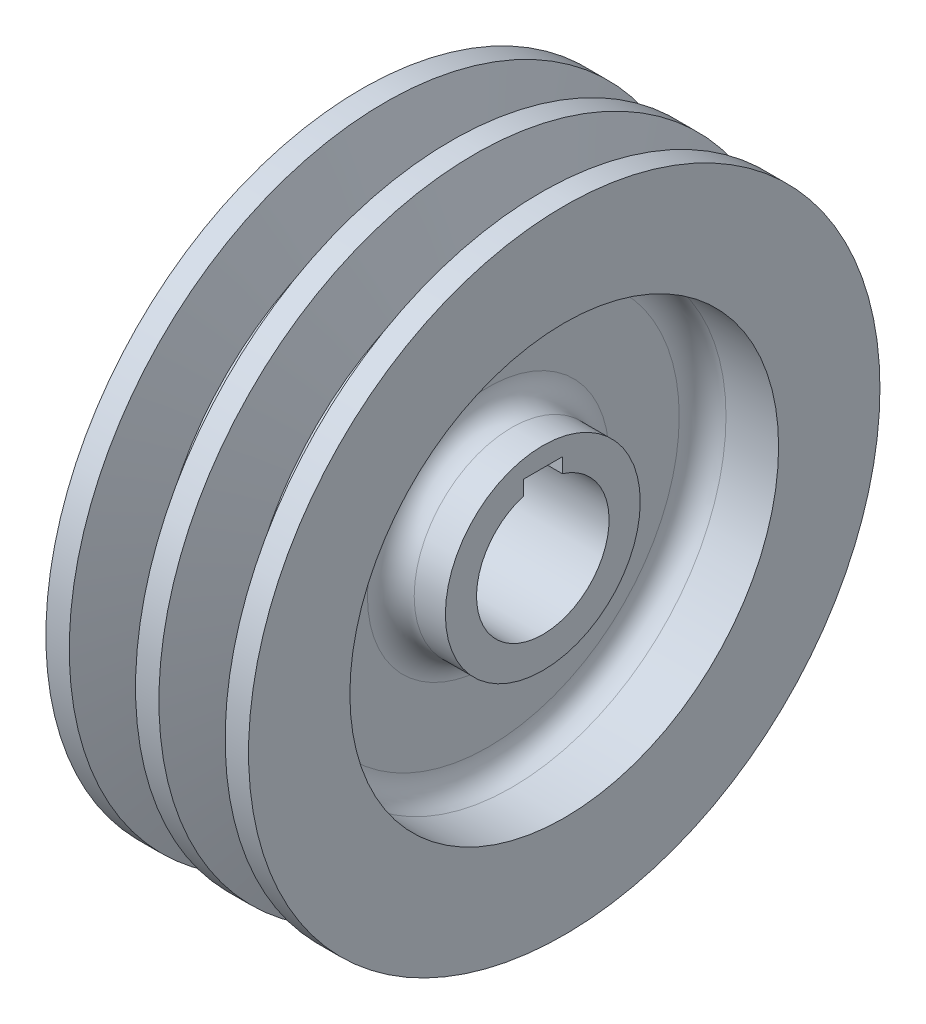
ISO-10303-21;
HEADER;
FILE_DESCRIPTION(('STEP AP214'),'2;1');
FILE_NAME('part.step','',(''),(''),'','','');
FILE_SCHEMA(('AUTOMOTIVE_DESIGN { 1 0 10303 214 1 1 1 1 }'));
ENDSEC;
DATA;
#1=APPLICATION_CONTEXT('core data for automotive mechanical design processes');
#2=APPLICATION_PROTOCOL_DEFINITION('international standard','automotive_design',2000,#1);
#3=PRODUCT_CONTEXT('',#1,'mechanical');
#4=PRODUCT('Part','Part','',(#3));
#5=PRODUCT_RELATED_PRODUCT_CATEGORY('part','',(#4));
#6=PRODUCT_DEFINITION_FORMATION('','',#4);
#7=PRODUCT_DEFINITION_CONTEXT('part definition',#1,'design');
#8=PRODUCT_DEFINITION('design','',#6,#7);
#9=PRODUCT_DEFINITION_SHAPE('','',#8);
#10=(LENGTH_UNIT() NAMED_UNIT(*) SI_UNIT(.MILLI.,.METRE.));
#11=(NAMED_UNIT(*) PLANE_ANGLE_UNIT() SI_UNIT($,.RADIAN.));
#12=(NAMED_UNIT(*) SI_UNIT($,.STERADIAN.) SOLID_ANGLE_UNIT());
#13=UNCERTAINTY_MEASURE_WITH_UNIT(LENGTH_MEASURE(1.E-05),#10,'distance_accuracy_value','');
#14=(GEOMETRIC_REPRESENTATION_CONTEXT(3) GLOBAL_UNCERTAINTY_ASSIGNED_CONTEXT((#13)) GLOBAL_UNIT_ASSIGNED_CONTEXT((#10,
#11,#12)) REPRESENTATION_CONTEXT('',''));
#15=CARTESIAN_POINT('',(0.,0.,0.));
#16=DIRECTION('',(0.,0.,1.));
#17=DIRECTION('',(1.,0.,0.));
#18=AXIS2_PLACEMENT_3D('',#15,#16,#17);
#19=CARTESIAN_POINT('',(52.,0.,0.));
#20=DIRECTION('',(-1.,0.,0.));
#21=DIRECTION('',(0.,0.,1.));
#22=AXIS2_PLACEMENT_3D('',#19,#20,#21);
#23=PLANE('',#22);
#24=CARTESIAN_POINT('',(52.,0.,0.));
#25=DIRECTION('',(1.,0.,0.));
#26=DIRECTION('',(0.,0.,-1.));
#27=AXIS2_PLACEMENT_3D('',#24,#25,#26);
#28=CIRCLE('',#27,55.);
#29=CARTESIAN_POINT('',(52.,0.,-55.));
#30=VERTEX_POINT('',#29);
#31=EDGE_CURVE('E135',#30,#30,#28,.T.);
#32=ORIENTED_EDGE('',*,*,#31,.F.);
#33=EDGE_LOOP('',(#32));
#34=FACE_BOUND('',#33,.T.);
#35=CARTESIAN_POINT('',(52.,0.,0.));
#36=DIRECTION('',(1.,0.,0.));
#37=DIRECTION('',(0.,0.,-1.));
#38=AXIS2_PLACEMENT_3D('',#35,#36,#37);
#39=CIRCLE('',#38,81.);
#40=CARTESIAN_POINT('',(52.,0.,-81.));
#41=VERTEX_POINT('',#40);
#42=EDGE_CURVE('E162',#41,#41,#39,.T.);
#43=ORIENTED_EDGE('',*,*,#42,.T.);
#44=EDGE_LOOP('',(#43));
#45=FACE_BOUND('',#44,.T.);
#46=ADVANCED_FACE('F50',(#34,#45),#23,.F.);
#47=CARTESIAN_POINT('',(52.,0.,0.));
#48=DIRECTION('',(1.,0.,0.));
#49=DIRECTION('',(0.,0.,-1.));
#50=AXIS2_PLACEMENT_3D('',#47,#48,#49);
#51=CYLINDRICAL_SURFACE('',#50,81.);
#52=ORIENTED_EDGE('',*,*,#42,.F.);
#53=EDGE_LOOP('',(#52));
#54=FACE_BOUND('',#53,.T.);
#55=CARTESIAN_POINT('',(46.,0.,0.));
#56=DIRECTION('',(1.,0.,0.));
#57=DIRECTION('',(0.,0.,-1.));
#58=AXIS2_PLACEMENT_3D('',#55,#56,#57);
#59=CIRCLE('',#58,81.);
#60=CARTESIAN_POINT('',(46.,0.,-81.));
#61=VERTEX_POINT('',#60);
#62=EDGE_CURVE('E158',#61,#61,#59,.T.);
#63=ORIENTED_EDGE('',*,*,#62,.T.);
#64=EDGE_LOOP('',(#63));
#65=FACE_BOUND('',#64,.T.);
#66=ADVANCED_FACE('F199',(#54,#65),#51,.T.);
#67=CARTESIAN_POINT('',(46.,0.,0.));
#68=DIRECTION('',(1.,0.,0.));
#69=DIRECTION('',(0.,0.,-1.));
#70=AXIS2_PLACEMENT_3D('',#67,#68,#69);
#71=CONICAL_SURFACE('',#70,81.,1.27409035395586);
#72=CARTESIAN_POINT('',(41.0300591318367,0.,0.));
#73=DIRECTION('',(1.,0.,0.));
#74=DIRECTION('',(0.,0.,-1.));
#75=AXIS2_PLACEMENT_3D('',#72,#73,#74);
#76=CIRCLE('',#75,64.7440558976569);
#77=CARTESIAN_POINT('',(41.0300591318367,0.,-64.7440558976569));
#78=VERTEX_POINT('',#77);
#79=EDGE_CURVE('E156',#78,#78,#76,.T.);
#80=ORIENTED_EDGE('',*,*,#79,.T.);
#81=EDGE_LOOP('',(#80));
#82=FACE_BOUND('',#81,.T.);
#83=ORIENTED_EDGE('',*,*,#62,.F.);
#84=EDGE_LOOP('',(#83));
#85=FACE_BOUND('',#84,.T.);
#86=ADVANCED_FACE('F210',(#82,#85),#71,.T.);
#87=CARTESIAN_POINT('',(52.,0.,0.));
#88=DIRECTION('',(1.,0.,0.));
#89=DIRECTION('',(0.,0.,-1.));
#90=AXIS2_PLACEMENT_3D('',#87,#88,#89);
#91=CYLINDRICAL_SURFACE('',#90,64.7440558976569);
#92=ORIENTED_EDGE('',*,*,#79,.F.);
#93=EDGE_LOOP('',(#92));
#94=FACE_BOUND('',#93,.T.);
#95=CARTESIAN_POINT('',(33.9699408681632,0.,0.));
#96=DIRECTION('',(1.,0.,0.));
#97=DIRECTION('',(0.,0.,-1.));
#98=AXIS2_PLACEMENT_3D('',#95,#96,#97);
#99=CIRCLE('',#98,64.7440558976569);
#100=CARTESIAN_POINT('',(33.9699408681632,0.,-64.7440558976569));
#101=VERTEX_POINT('',#100);
#102=EDGE_CURVE('E151',#101,#101,#99,.T.);
#103=ORIENTED_EDGE('',*,*,#102,.T.);
#104=EDGE_LOOP('',(#103));
#105=FACE_BOUND('',#104,.T.);
#106=ADVANCED_FACE('F277',(#94,#105),#91,.T.);
#107=CARTESIAN_POINT('',(29.,0.,0.));
#108=DIRECTION('',(-1.,0.,0.));
#109=DIRECTION('',(0.,0.,1.));
#110=AXIS2_PLACEMENT_3D('',#107,#108,#109);
#111=CONICAL_SURFACE('',#110,81.,1.27409035395586);
#112=ORIENTED_EDGE('',*,*,#102,.F.);
#113=EDGE_LOOP('',(#112));
#114=FACE_BOUND('',#113,.T.);
#115=CARTESIAN_POINT('',(29.,0.,0.));
#116=DIRECTION('',(1.,0.,0.));
#117=DIRECTION('',(0.,0.,-1.));
#118=AXIS2_PLACEMENT_3D('',#115,#116,#117);
#119=CIRCLE('',#118,81.);
#120=CARTESIAN_POINT('',(29.,0.,-81.));
#121=VERTEX_POINT('',#120);
#122=EDGE_CURVE('E148',#121,#121,#119,.T.);
#123=ORIENTED_EDGE('',*,*,#122,.T.);
#124=EDGE_LOOP('',(#123));
#125=FACE_BOUND('',#124,.T.);
#126=ADVANCED_FACE('F275',(#114,#125),#111,.T.);
#127=CARTESIAN_POINT('',(52.,0.,0.));
#128=DIRECTION('',(1.,0.,0.));
#129=DIRECTION('',(0.,0.,-1.));
#130=AXIS2_PLACEMENT_3D('',#127,#128,#129);
#131=CYLINDRICAL_SURFACE('',#130,81.);
#132=ORIENTED_EDGE('',*,*,#122,.F.);
#133=EDGE_LOOP('',(#132));
#134=FACE_BOUND('',#133,.T.);
#135=CARTESIAN_POINT('',(23.,0.,0.));
#136=DIRECTION('',(1.,0.,0.));
#137=DIRECTION('',(0.,0.,-1.));
#138=AXIS2_PLACEMENT_3D('',#135,#136,#137);
#139=CIRCLE('',#138,81.);
#140=CARTESIAN_POINT('',(23.,0.,-81.));
#141=VERTEX_POINT('',#140);
#142=EDGE_CURVE('E150',#141,#141,#139,.T.);
#143=ORIENTED_EDGE('',*,*,#142,.T.);
#144=EDGE_LOOP('',(#143));
#145=FACE_BOUND('',#144,.T.);
#146=ADVANCED_FACE('F269',(#134,#145),#131,.T.);
#147=CARTESIAN_POINT('',(23.,0.,0.));
#148=DIRECTION('',(1.,0.,0.));
#149=DIRECTION('',(0.,0.,-1.));
#150=AXIS2_PLACEMENT_3D('',#147,#148,#149);
#151=CONICAL_SURFACE('',#150,81.,1.27409035395586);
#152=CARTESIAN_POINT('',(18.0300591318367,0.,0.));
#153=DIRECTION('',(1.,0.,0.));
#154=DIRECTION('',(0.,0.,-1.));
#155=AXIS2_PLACEMENT_3D('',#152,#153,#154);
#156=CIRCLE('',#155,64.7440558976569);
#157=CARTESIAN_POINT('',(18.0300591318367,0.,-64.7440558976569));
#158=VERTEX_POINT('',#157);
#159=EDGE_CURVE('E144',#158,#158,#156,.T.);
#160=ORIENTED_EDGE('',*,*,#159,.T.);
#161=EDGE_LOOP('',(#160));
#162=FACE_BOUND('',#161,.T.);
#163=ORIENTED_EDGE('',*,*,#142,.F.);
#164=EDGE_LOOP('',(#163));
#165=FACE_BOUND('',#164,.T.);
#166=ADVANCED_FACE('F264',(#162,#165),#151,.T.);
#167=CARTESIAN_POINT('',(52.,0.,0.));
#168=DIRECTION('',(1.,0.,0.));
#169=DIRECTION('',(0.,0.,-1.));
#170=AXIS2_PLACEMENT_3D('',#167,#168,#169);
#171=CYLINDRICAL_SURFACE('',#170,64.7440558976569);
#172=ORIENTED_EDGE('',*,*,#159,.F.);
#173=EDGE_LOOP('',(#172));
#174=FACE_BOUND('',#173,.T.);
#175=CARTESIAN_POINT('',(10.9699408681632,0.,0.));
#176=DIRECTION('',(1.,0.,0.));
#177=DIRECTION('',(0.,0.,-1.));
#178=AXIS2_PLACEMENT_3D('',#175,#176,#177);
#179=CIRCLE('',#178,64.7440558976569);
#180=CARTESIAN_POINT('',(10.9699408681632,0.,-64.7440558976569));
#181=VERTEX_POINT('',#180);
#182=EDGE_CURVE('E142',#181,#181,#179,.T.);
#183=ORIENTED_EDGE('',*,*,#182,.T.);
#184=EDGE_LOOP('',(#183));
#185=FACE_BOUND('',#184,.T.);
#186=ADVANCED_FACE('F258',(#174,#185),#171,.T.);
#187=CARTESIAN_POINT('',(6.,0.,0.));
#188=DIRECTION('',(-1.,0.,0.));
#189=DIRECTION('',(0.,0.,1.));
#190=AXIS2_PLACEMENT_3D('',#187,#188,#189);
#191=CONICAL_SURFACE('',#190,81.,1.27409035395586);
#192=ORIENTED_EDGE('',*,*,#182,.F.);
#193=EDGE_LOOP('',(#192));
#194=FACE_BOUND('',#193,.T.);
#195=CARTESIAN_POINT('',(6.,0.,0.));
#196=DIRECTION('',(1.,0.,0.));
#197=DIRECTION('',(0.,0.,-1.));
#198=AXIS2_PLACEMENT_3D('',#195,#196,#197);
#199=CIRCLE('',#198,81.);
#200=CARTESIAN_POINT('',(6.,0.,-81.));
#201=VERTEX_POINT('',#200);
#202=EDGE_CURVE('E139',#201,#201,#199,.T.);
#203=ORIENTED_EDGE('',*,*,#202,.T.);
#204=EDGE_LOOP('',(#203));
#205=FACE_BOUND('',#204,.T.);
#206=ADVANCED_FACE('F257',(#194,#205),#191,.T.);
#207=CARTESIAN_POINT('',(52.,0.,0.));
#208=DIRECTION('',(1.,0.,0.));
#209=DIRECTION('',(0.,0.,-1.));
#210=AXIS2_PLACEMENT_3D('',#207,#208,#209);
#211=CYLINDRICAL_SURFACE('',#210,81.);
#212=ORIENTED_EDGE('',*,*,#202,.F.);
#213=EDGE_LOOP('',(#212));
#214=FACE_BOUND('',#213,.T.);
#215=CARTESIAN_POINT('',(0.,0.,0.));
#216=DIRECTION('',(1.,0.,0.));
#217=DIRECTION('',(0.,0.,-1.));
#218=AXIS2_PLACEMENT_3D('',#215,#216,#217);
#219=CIRCLE('',#218,81.);
#220=CARTESIAN_POINT('',(0.,0.,-81.));
#221=VERTEX_POINT('',#220);
#222=EDGE_CURVE('E132',#221,#221,#219,.T.);
#223=ORIENTED_EDGE('',*,*,#222,.T.);
#224=EDGE_LOOP('',(#223));
#225=FACE_BOUND('',#224,.T.);
#226=ADVANCED_FACE('F254',(#214,#225),#211,.T.);
#227=CARTESIAN_POINT('',(0.,0.,0.));
#228=DIRECTION('',(1.,0.,0.));
#229=DIRECTION('',(0.,0.,-1.));
#230=AXIS2_PLACEMENT_3D('',#227,#228,#229);
#231=PLANE('',#230);
#232=CARTESIAN_POINT('',(0.,0.,0.));
#233=DIRECTION('',(-1.,0.,0.));
#234=DIRECTION('',(0.,0.,1.));
#235=AXIS2_PLACEMENT_3D('',#232,#233,#234);
#236=CIRCLE('',#235,55.);
#237=CARTESIAN_POINT('',(0.,0.,55.));
#238=VERTEX_POINT('',#237);
#239=EDGE_CURVE('E126',#238,#238,#236,.T.);
#240=ORIENTED_EDGE('',*,*,#239,.F.);
#241=EDGE_LOOP('',(#240));
#242=FACE_BOUND('',#241,.T.);
#243=ORIENTED_EDGE('',*,*,#222,.F.);
#244=EDGE_LOOP('',(#243));
#245=FACE_BOUND('',#244,.T.);
#246=ADVANCED_FACE('F249',(#242,#245),#231,.F.);
#247=CARTESIAN_POINT('',(32.5,0.,0.));
#248=DIRECTION('',(1.,0.,0.));
#249=DIRECTION('',(0.,0.,-1.));
#250=AXIS2_PLACEMENT_3D('',#247,#248,#249);
#251=CYLINDRICAL_SURFACE('',#250,55.);
#252=CARTESIAN_POINT('',(38.5,0.,0.));
#253=DIRECTION('',(1.,0.,0.));
#254=DIRECTION('',(0.,0.,-1.));
#255=AXIS2_PLACEMENT_3D('',#252,#253,#254);
#256=CIRCLE('',#255,55.);
#257=CARTESIAN_POINT('',(38.5,0.,-55.));
#258=VERTEX_POINT('',#257);
#259=EDGE_CURVE('E166',#258,#258,#256,.F.);
#260=ORIENTED_EDGE('',*,*,#259,.T.);
#261=EDGE_LOOP('',(#260));
#262=FACE_BOUND('',#261,.T.);
#263=ORIENTED_EDGE('',*,*,#31,.T.);
#264=EDGE_LOOP('',(#263));
#265=FACE_BOUND('',#264,.T.);
#266=ADVANCED_FACE('F246',(#262,#265),#251,.F.);
#267=CARTESIAN_POINT('',(32.5,0.,0.));
#268=DIRECTION('',(1.,0.,0.));
#269=DIRECTION('',(0.,0.,-1.));
#270=AXIS2_PLACEMENT_3D('',#267,#268,#269);
#271=PLANE('',#270);
#272=CARTESIAN_POINT('',(32.5,0.,0.));
#273=DIRECTION('',(1.,0.,0.));
#274=DIRECTION('',(0.,0.,-1.));
#275=AXIS2_PLACEMENT_3D('',#272,#273,#274);
#276=CIRCLE('',#275,31.);
#277=CARTESIAN_POINT('',(32.5,0.,-31.));
#278=VERTEX_POINT('',#277);
#279=EDGE_CURVE('E179',#278,#278,#276,.F.);
#280=ORIENTED_EDGE('',*,*,#279,.T.);
#281=EDGE_LOOP('',(#280));
#282=FACE_BOUND('',#281,.T.);
#283=CARTESIAN_POINT('',(32.5,0.,0.));
#284=DIRECTION('',(1.,0.,0.));
#285=DIRECTION('',(0.,0.,-1.));
#286=AXIS2_PLACEMENT_3D('',#283,#284,#285);
#287=CIRCLE('',#286,49.);
#288=CARTESIAN_POINT('',(32.5,0.,-49.));
#289=VERTEX_POINT('',#288);
#290=EDGE_CURVE('E164',#289,#289,#287,.T.);
#291=ORIENTED_EDGE('',*,*,#290,.T.);
#292=EDGE_LOOP('',(#291));
#293=FACE_BOUND('',#292,.T.);
#294=ADVANCED_FACE('F239',(#282,#293),#271,.T.);
#295=CARTESIAN_POINT('',(19.5,0.,0.));
#296=DIRECTION('',(-1.,0.,0.));
#297=DIRECTION('',(0.,0.,1.));
#298=AXIS2_PLACEMENT_3D('',#295,#296,#297);
#299=CYLINDRICAL_SURFACE('',#298,55.);
#300=CARTESIAN_POINT('',(13.5,0.,0.));
#301=DIRECTION('',(-1.,0.,0.));
#302=DIRECTION('',(0.,0.,1.));
#303=AXIS2_PLACEMENT_3D('',#300,#301,#302);
#304=CIRCLE('',#303,55.);
#305=CARTESIAN_POINT('',(13.5,0.,55.));
#306=VERTEX_POINT('',#305);
#307=EDGE_CURVE('E172',#306,#306,#304,.F.);
#308=ORIENTED_EDGE('',*,*,#307,.T.);
#309=EDGE_LOOP('',(#308));
#310=FACE_BOUND('',#309,.T.);
#311=ORIENTED_EDGE('',*,*,#239,.T.);
#312=EDGE_LOOP('',(#311));
#313=FACE_BOUND('',#312,.T.);
#314=ADVANCED_FACE('F233',(#310,#313),#299,.F.);
#315=CARTESIAN_POINT('',(19.5,0.,0.));
#316=DIRECTION('',(-1.,0.,0.));
#317=DIRECTION('',(0.,0.,1.));
#318=AXIS2_PLACEMENT_3D('',#315,#316,#317);
#319=PLANE('',#318);
#320=CARTESIAN_POINT('',(19.5,0.,0.));
#321=DIRECTION('',(-1.,0.,0.));
#322=DIRECTION('',(0.,0.,1.));
#323=AXIS2_PLACEMENT_3D('',#320,#321,#322);
#324=CIRCLE('',#323,31.);
#325=CARTESIAN_POINT('',(19.5,0.,31.));
#326=VERTEX_POINT('',#325);
#327=EDGE_CURVE('E11',#326,#326,#324,.F.);
#328=ORIENTED_EDGE('',*,*,#327,.T.);
#329=EDGE_LOOP('',(#328));
#330=FACE_BOUND('',#329,.T.);
#331=CARTESIAN_POINT('',(19.5,0.,0.));
#332=DIRECTION('',(-1.,0.,0.));
#333=DIRECTION('',(0.,0.,1.));
#334=AXIS2_PLACEMENT_3D('',#331,#332,#333);
#335=CIRCLE('',#334,49.);
#336=CARTESIAN_POINT('',(19.5,0.,49.));
#337=VERTEX_POINT('',#336);
#338=EDGE_CURVE('E171',#337,#337,#335,.T.);
#339=ORIENTED_EDGE('',*,*,#338,.T.);
#340=EDGE_LOOP('',(#339));
#341=FACE_BOUND('',#340,.T.);
#342=ADVANCED_FACE('F226',(#330,#341),#319,.T.);
#343=CARTESIAN_POINT('',(46.5,0.,0.));
#344=DIRECTION('',(-1.,0.,0.));
#345=DIRECTION('',(0.,0.,1.));
#346=AXIS2_PLACEMENT_3D('',#343,#344,#345);
#347=CYLINDRICAL_SURFACE('',#346,25.);
#348=CARTESIAN_POINT('',(38.5,0.,0.));
#349=DIRECTION('',(1.,0.,0.));
#350=DIRECTION('',(0.,0.,-1.));
#351=AXIS2_PLACEMENT_3D('',#348,#349,#350);
#352=CIRCLE('',#351,25.);
#353=CARTESIAN_POINT('',(38.5,0.,-25.));
#354=VERTEX_POINT('',#353);
#355=EDGE_CURVE('E180',#354,#354,#352,.T.);
#356=ORIENTED_EDGE('',*,*,#355,.T.);
#357=EDGE_LOOP('',(#356));
#358=FACE_BOUND('',#357,.T.);
#359=CARTESIAN_POINT('',(46.5,0.,0.));
#360=DIRECTION('',(1.,0.,0.));
#361=DIRECTION('',(0.,0.,-1.));
#362=AXIS2_PLACEMENT_3D('',#359,#360,#361);
#363=CIRCLE('',#362,25.);
#364=CARTESIAN_POINT('',(46.5,0.,-25.));
#365=VERTEX_POINT('',#364);
#366=EDGE_CURVE('E127',#365,#365,#363,.T.);
#367=ORIENTED_EDGE('',*,*,#366,.F.);
#368=EDGE_LOOP('',(#367));
#369=FACE_BOUND('',#368,.T.);
#370=ADVANCED_FACE('F229',(#358,#369),#347,.T.);
#371=CARTESIAN_POINT('',(46.5,0.,0.));
#372=DIRECTION('',(1.,0.,0.));
#373=DIRECTION('',(0.,0.,-1.));
#374=AXIS2_PLACEMENT_3D('',#371,#372,#373);
#375=PLANE('',#374);
#376=DIRECTION('',(0.,0.,1.));
#377=VECTOR('',#376,1.);
#378=CARTESIAN_POINT('',(46.5,20.,0.));
#379=LINE('',#378,#377);
#380=CARTESIAN_POINT('',(46.5,20.,-5.));
#381=VERTEX_POINT('',#380);
#382=CARTESIAN_POINT('',(46.5,20.,5.));
#383=VERTEX_POINT('',#382);
#384=EDGE_CURVE('E122',#381,#383,#379,.T.);
#385=ORIENTED_EDGE('',*,*,#384,.F.);
#386=DIRECTION('',(0.,1.,0.));
#387=VECTOR('',#386,1.);
#388=CARTESIAN_POINT('',(46.5,0.,-5.));
#389=LINE('',#388,#387);
#390=CARTESIAN_POINT('',(46.5,16.2480768092719,-5.));
#391=VERTEX_POINT('',#390);
#392=EDGE_CURVE('E112',#391,#381,#389,.T.);
#393=ORIENTED_EDGE('',*,*,#392,.F.);
#394=CARTESIAN_POINT('',(46.5,0.,0.));
#395=DIRECTION('',(1.,0.,0.));
#396=DIRECTION('',(0.,0.,-1.));
#397=AXIS2_PLACEMENT_3D('',#394,#395,#396);
#398=CIRCLE('',#397,17.);
#399=CARTESIAN_POINT('',(46.5,16.2480768092719,5.));
#400=VERTEX_POINT('',#399);
#401=EDGE_CURVE('E93',#400,#391,#398,.T.);
#402=ORIENTED_EDGE('',*,*,#401,.F.);
#403=DIRECTION('',(0.,-1.,0.));
#404=VECTOR('',#403,1.);
#405=CARTESIAN_POINT('',(46.5,0.,4.99999999999999));
#406=LINE('',#405,#404);
#407=EDGE_CURVE('E118',#383,#400,#406,.T.);
#408=ORIENTED_EDGE('',*,*,#407,.F.);
#409=EDGE_LOOP('',(#385,#393,#402,#408));
#410=FACE_BOUND('',#409,.T.);
#411=ORIENTED_EDGE('',*,*,#366,.T.);
#412=EDGE_LOOP('',(#411));
#413=FACE_BOUND('',#412,.T.);
#414=ADVANCED_FACE('F240',(#410,#413),#375,.T.);
#415=CARTESIAN_POINT('',(5.5,0.,0.));
#416=DIRECTION('',(1.,0.,0.));
#417=DIRECTION('',(0.,0.,-1.));
#418=AXIS2_PLACEMENT_3D('',#415,#416,#417);
#419=CYLINDRICAL_SURFACE('',#418,25.);
#420=CARTESIAN_POINT('',(13.5,0.,0.));
#421=DIRECTION('',(-1.,0.,0.));
#422=DIRECTION('',(0.,0.,1.));
#423=AXIS2_PLACEMENT_3D('',#420,#421,#422);
#424=CIRCLE('',#423,25.);
#425=CARTESIAN_POINT('',(13.5,0.,25.));
#426=VERTEX_POINT('',#425);
#427=EDGE_CURVE('E54',#426,#426,#424,.T.);
#428=ORIENTED_EDGE('',*,*,#427,.T.);
#429=EDGE_LOOP('',(#428));
#430=FACE_BOUND('',#429,.T.);
#431=CARTESIAN_POINT('',(5.5,0.,0.));
#432=DIRECTION('',(-1.,0.,0.));
#433=DIRECTION('',(0.,0.,1.));
#434=AXIS2_PLACEMENT_3D('',#431,#432,#433);
#435=CIRCLE('',#434,25.);
#436=CARTESIAN_POINT('',(5.5,0.,25.));
#437=VERTEX_POINT('',#436);
#438=EDGE_CURVE('E124',#437,#437,#435,.T.);
#439=ORIENTED_EDGE('',*,*,#438,.F.);
#440=EDGE_LOOP('',(#439));
#441=FACE_BOUND('',#440,.T.);
#442=ADVANCED_FACE('F184',(#430,#441),#419,.T.);
#443=CARTESIAN_POINT('',(5.5,0.,0.));
#444=DIRECTION('',(-1.,0.,0.));
#445=DIRECTION('',(0.,0.,1.));
#446=AXIS2_PLACEMENT_3D('',#443,#444,#445);
#447=PLANE('',#446);
#448=DIRECTION('',(0.,0.,-1.));
#449=VECTOR('',#448,1.);
#450=CARTESIAN_POINT('',(5.5,20.,0.));
#451=LINE('',#450,#449);
#452=CARTESIAN_POINT('',(5.5,20.,5.));
#453=VERTEX_POINT('',#452);
#454=CARTESIAN_POINT('',(5.5,20.,-5.));
#455=VERTEX_POINT('',#454);
#456=EDGE_CURVE('E67',#453,#455,#451,.T.);
#457=ORIENTED_EDGE('',*,*,#456,.F.);
#458=DIRECTION('',(0.,1.,0.));
#459=VECTOR('',#458,1.);
#460=CARTESIAN_POINT('',(5.5,20.,5.));
#461=LINE('',#460,#459);
#462=CARTESIAN_POINT('',(5.5,16.2480768092719,5.));
#463=VERTEX_POINT('',#462);
#464=EDGE_CURVE('E110',#463,#453,#461,.T.);
#465=ORIENTED_EDGE('',*,*,#464,.F.);
#466=CARTESIAN_POINT('',(5.5,0.,0.));
#467=DIRECTION('',(-1.,0.,0.));
#468=DIRECTION('',(0.,0.,1.));
#469=AXIS2_PLACEMENT_3D('',#466,#467,#468);
#470=CIRCLE('',#469,17.);
#471=CARTESIAN_POINT('',(5.5,16.2480768092719,-5.));
#472=VERTEX_POINT('',#471);
#473=EDGE_CURVE('E91',#472,#463,#470,.T.);
#474=ORIENTED_EDGE('',*,*,#473,.F.);
#475=DIRECTION('',(0.,-1.,0.));
#476=VECTOR('',#475,1.);
#477=CARTESIAN_POINT('',(5.5,16.2480768092719,-5.));
#478=LINE('',#477,#476);
#479=EDGE_CURVE('E99',#455,#472,#478,.T.);
#480=ORIENTED_EDGE('',*,*,#479,.F.);
#481=EDGE_LOOP('',(#457,#465,#474,#480));
#482=FACE_BOUND('',#481,.T.);
#483=ORIENTED_EDGE('',*,*,#438,.T.);
#484=EDGE_LOOP('',(#483));
#485=FACE_BOUND('',#484,.T.);
#486=ADVANCED_FACE('F104',(#482,#485),#447,.T.);
#487=CARTESIAN_POINT('',(94.5,20.,0.));
#488=DIRECTION('',(0.,1.,0.));
#489=DIRECTION('',(0.,0.,1.));
#490=AXIS2_PLACEMENT_3D('',#487,#488,#489);
#491=PLANE('',#490);
#492=ORIENTED_EDGE('',*,*,#384,.T.);
#493=DIRECTION('',(-1.,0.,0.));
#494=VECTOR('',#493,1.);
#495=CARTESIAN_POINT('',(94.5,20.,5.));
#496=LINE('',#495,#494);
#497=EDGE_CURVE('E115',#383,#453,#496,.T.);
#498=ORIENTED_EDGE('',*,*,#497,.T.);
#499=ORIENTED_EDGE('',*,*,#456,.T.);
#500=DIRECTION('',(-1.,0.,0.));
#501=VECTOR('',#500,1.);
#502=CARTESIAN_POINT('',(94.5,20.,-5.));
#503=LINE('',#502,#501);
#504=EDGE_CURVE('E97',#381,#455,#503,.T.);
#505=ORIENTED_EDGE('',*,*,#504,.F.);
#506=EDGE_LOOP('',(#492,#498,#499,#505));
#507=FACE_BOUND('',#506,.T.);
#508=ADVANCED_FACE('F392',(#507),#491,.F.);
#509=CARTESIAN_POINT('',(94.5,20.,5.));
#510=DIRECTION('',(0.,0.,1.));
#511=DIRECTION('',(0.,-1.,0.));
#512=AXIS2_PLACEMENT_3D('',#509,#510,#511);
#513=PLANE('',#512);
#514=ORIENTED_EDGE('',*,*,#407,.T.);
#515=DIRECTION('',(-1.,0.,0.));
#516=VECTOR('',#515,1.);
#517=CARTESIAN_POINT('',(94.5,16.2480768092719,5.));
#518=LINE('',#517,#516);
#519=EDGE_CURVE('E98',#400,#463,#518,.T.);
#520=ORIENTED_EDGE('',*,*,#519,.T.);
#521=ORIENTED_EDGE('',*,*,#464,.T.);
#522=ORIENTED_EDGE('',*,*,#497,.F.);
#523=EDGE_LOOP('',(#514,#520,#521,#522));
#524=FACE_BOUND('',#523,.T.);
#525=ADVANCED_FACE('F403',(#524),#513,.F.);
#526=CARTESIAN_POINT('',(94.5,0.,0.));
#527=DIRECTION('',(-1.,0.,0.));
#528=DIRECTION('',(0.,0.,1.));
#529=AXIS2_PLACEMENT_3D('',#526,#527,#528);
#530=CYLINDRICAL_SURFACE('',#529,17.);
#531=ORIENTED_EDGE('',*,*,#401,.T.);
#532=DIRECTION('',(-1.,0.,0.));
#533=VECTOR('',#532,1.);
#534=CARTESIAN_POINT('',(94.5,16.2480768092719,-5.));
#535=LINE('',#534,#533);
#536=EDGE_CURVE('E65',#391,#472,#535,.T.);
#537=ORIENTED_EDGE('',*,*,#536,.T.);
#538=ORIENTED_EDGE('',*,*,#473,.T.);
#539=ORIENTED_EDGE('',*,*,#519,.F.);
#540=EDGE_LOOP('',(#531,#537,#538,#539));
#541=FACE_BOUND('',#540,.T.);
#542=ADVANCED_FACE('F86',(#541),#530,.F.);
#543=CARTESIAN_POINT('',(94.5,16.2480768092719,-5.));
#544=DIRECTION('',(0.,0.,-1.));
#545=DIRECTION('',(-1.,0.,0.));
#546=AXIS2_PLACEMENT_3D('',#543,#544,#545);
#547=PLANE('',#546);
#548=ORIENTED_EDGE('',*,*,#392,.T.);
#549=ORIENTED_EDGE('',*,*,#504,.T.);
#550=ORIENTED_EDGE('',*,*,#479,.T.);
#551=ORIENTED_EDGE('',*,*,#536,.F.);
#552=EDGE_LOOP('',(#548,#549,#550,#551));
#553=FACE_BOUND('',#552,.T.);
#554=ADVANCED_FACE('F103',(#553),#547,.F.);
#555=CARTESIAN_POINT('',(38.5,0.,0.));
#556=DIRECTION('',(1.,0.,0.));
#557=DIRECTION('',(0.,0.,-1.));
#558=AXIS2_PLACEMENT_3D('',#555,#556,#557);
#559=TOROIDAL_SURFACE('',#558,49.,6.);
#560=ORIENTED_EDGE('',*,*,#259,.F.);
#561=EDGE_LOOP('',(#560));
#562=FACE_BOUND('',#561,.T.);
#563=ORIENTED_EDGE('',*,*,#290,.F.);
#564=EDGE_LOOP('',(#563));
#565=FACE_BOUND('',#564,.T.);
#566=ADVANCED_FACE('F211',(#562,#565),#559,.F.);
#567=CARTESIAN_POINT('',(13.5,0.,0.));
#568=DIRECTION('',(-1.,0.,0.));
#569=DIRECTION('',(0.,0.,1.));
#570=AXIS2_PLACEMENT_3D('',#567,#568,#569);
#571=TOROIDAL_SURFACE('',#570,49.,6.);
#572=ORIENTED_EDGE('',*,*,#307,.F.);
#573=EDGE_LOOP('',(#572));
#574=FACE_BOUND('',#573,.T.);
#575=ORIENTED_EDGE('',*,*,#338,.F.);
#576=EDGE_LOOP('',(#575));
#577=FACE_BOUND('',#576,.T.);
#578=ADVANCED_FACE('F193',(#574,#577),#571,.F.);
#579=CARTESIAN_POINT('',(38.5,0.,0.));
#580=DIRECTION('',(1.,0.,0.));
#581=DIRECTION('',(0.,0.,-1.));
#582=AXIS2_PLACEMENT_3D('',#579,#580,#581);
#583=TOROIDAL_SURFACE('',#582,31.,6.);
#584=ORIENTED_EDGE('',*,*,#279,.F.);
#585=EDGE_LOOP('',(#584));
#586=FACE_BOUND('',#585,.T.);
#587=ORIENTED_EDGE('',*,*,#355,.F.);
#588=EDGE_LOOP('',(#587));
#589=FACE_BOUND('',#588,.T.);
#590=ADVANCED_FACE('F186',(#586,#589),#583,.F.);
#591=CARTESIAN_POINT('',(13.5,0.,0.));
#592=DIRECTION('',(-1.,0.,0.));
#593=DIRECTION('',(0.,0.,1.));
#594=AXIS2_PLACEMENT_3D('',#591,#592,#593);
#595=TOROIDAL_SURFACE('',#594,31.,6.);
#596=ORIENTED_EDGE('',*,*,#327,.F.);
#597=EDGE_LOOP('',(#596));
#598=FACE_BOUND('',#597,.T.);
#599=ORIENTED_EDGE('',*,*,#427,.F.);
#600=EDGE_LOOP('',(#599));
#601=FACE_BOUND('',#600,.T.);
#602=ADVANCED_FACE('F47',(#598,#601),#595,.F.);
#603=CLOSED_SHELL('',(#46,#66,#86,#106,#126,#146,#166,#186,#206,#226,#246,#266,#294,#314,#342,
#370,#414,#442,#486,#508,#525,#542,#554,#566,#578,#590,#602));
#604=MANIFOLD_SOLID_BREP('B2',#603);
#605=ADVANCED_BREP_SHAPE_REPRESENTATION('',(#18,#604),#14);
#606=SHAPE_DEFINITION_REPRESENTATION(#9,#605);
ENDSEC;
END-ISO-10303-21;
